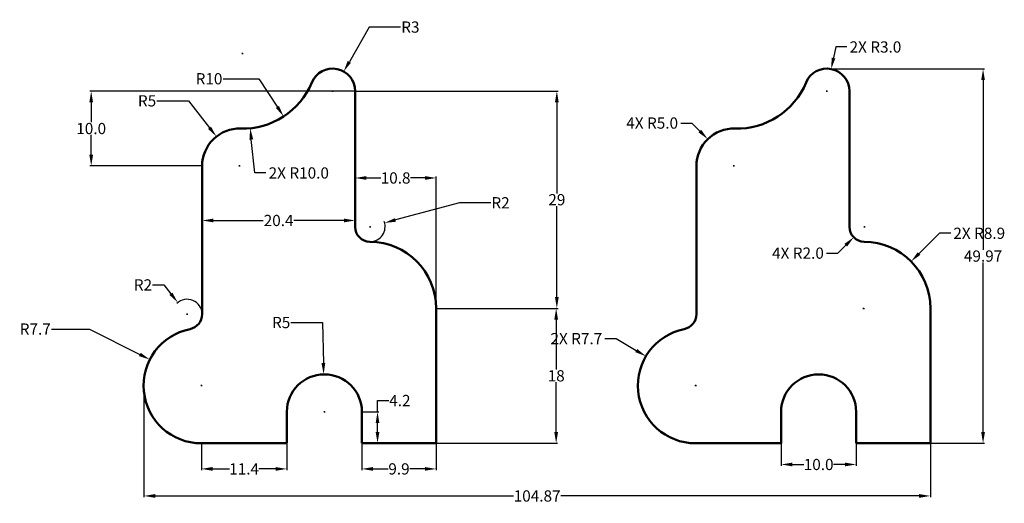
# Model space of a CAD drawing. Units: millimetres. Extents: x -11 to 121, y -3 to 61.
import ezdxf

# ---------------------------------------------------------------- set-up
doc = ezdxf.new("R2010")
doc.units = ezdxf.units.MM
doc.header["$MEASUREMENT"] = 0
doc.layers.add('M-DIMS', color=3, linetype='Continuous', lineweight=25)
doc.layers.add('M-OUTL', color=7, linetype='Continuous', lineweight=50)
doc.styles.get("Standard").update_dxf_attribs({"font": 'arial.ttf'})
doc.dimstyles.get("Standard").update_dxf_attribs({"dimtxt": 1.5, "dimasz": 1.5, "dimexe": 0.18, "dimexo": 0.0625, "dimgap": 0.09, "dimtad": 0, "dimtih": 1, "dimtoh": 1, "dimdec": 1, "dimdsep": 46, "dimtxsty": 'Standard', "dimcen": 0.09, "dimadec": 0, "dimazin": 0, "dimtfac": 1, "dimtdec": 1, "dimtofl": 0, "dimtmove": 0, "dimatfit": 3, "dimfxl": 1, "dimtolj": 1, "dimtzin": 0, "dimarcsym": 0})

# ---------------------------------------------------------------- blocks, each defined once
blk = doc.blocks.new('*D1')
at = {"layer": 'Defpoints', "color": 0, "transparency": 16777216}
for p in [(13.55, 4.95), (24.95, 4.95), (24.95, 1.53)]:
    blk.add_point(p, dxfattribs=at)
at = {"layer": 'M-DIMS', "color": 0, "lineweight": -2, "transparency": 16777216}
for p, q in [((13.55, 4.88), (13.55, 1.35)), ((24.95, 4.88), (24.95, 1.35)), ((15.05, 1.53), (17.29, 1.53)), ((23.45, 1.53), (21.22, 1.53))]:
    blk.add_line(p, q, dxfattribs=at)
at = {"layer": 'M-DIMS', "color": 0, "transparency": 16777216}
for points in [[(15.05, 1.78), (15.05, 1.28), (13.55, 1.53)], [(23.45, 1.78), (23.45, 1.28), (24.95, 1.53)]]:
    blk.add_solid(points, dxfattribs=at)
at = {"layer": 'M-DIMS', "color": 0, "transparency": 16777216, "insert": (19.25, 1.53), "char_height": 1.5, "attachment_point": 5}
blk.add_mtext('\\A1;11.4', dxfattribs=at)
blk = doc.blocks.new('*D2')
at = {"layer": 'Defpoints', "color": 0, "transparency": 16777216}
for p in [(34.95, 4.95), (44.85, 4.95), (44.85, 1.53)]:
    blk.add_point(p, dxfattribs=at)
at = {"layer": 'M-DIMS', "color": 0, "lineweight": -2, "transparency": 16777216}
for p, q in [((34.95, 4.88), (34.95, 1.35)), ((44.85, 4.88), (44.85, 1.35)), ((36.45, 1.53), (38.44, 1.53)), ((43.35, 1.53), (41.36, 1.53))]:
    blk.add_line(p, q, dxfattribs=at)
at = {"layer": 'M-DIMS', "color": 0, "transparency": 16777216}
for points in [[(36.45, 1.78), (36.45, 1.28), (34.95, 1.53)], [(43.35, 1.78), (43.35, 1.28), (44.85, 1.53)]]:
    blk.add_solid(points, dxfattribs=at)
at = {"layer": 'M-DIMS', "color": 0, "transparency": 16777216, "insert": (39.9, 1.53), "char_height": 1.5, "attachment_point": 5}
blk.add_mtext('\\A1;9.9', dxfattribs=at)
blk = doc.blocks.new('*D3')
at = {"layer": 'Defpoints', "color": 0, "transparency": 16777216}
for p in [(34.95, 9.15), (37.04, 9.15), (34.95, 4.95)]:
    blk.add_point(p, dxfattribs=at)
at = {"layer": 'M-DIMS', "color": 0, "lineweight": -2, "transparency": 16777216}
for p, q in [((37.04, 9.15), (37.04, 10.65)), ((37.04, 10.65), (38.54, 10.65)), ((35.01, 9.15), (37.22, 9.15)), ((37.04, 6.45), (37.04, 7.65)), ((35.01, 4.95), (37.22, 4.95))]:
    blk.add_line(p, q, dxfattribs=at)
at = {"layer": 'M-DIMS', "color": 0, "transparency": 16777216}
for points in [[(36.79, 7.65), (37.29, 7.65), (37.04, 9.15)], [(36.79, 6.45), (37.29, 6.45), (37.04, 4.95)]]:
    blk.add_solid(points, dxfattribs=at)
at = {"layer": 'M-DIMS', "color": 0, "transparency": 16777216, "insert": (40.02, 10.65), "char_height": 1.5, "attachment_point": 5}
blk.add_mtext('\\A1;4.2', dxfattribs=at)
blk = doc.blocks.new('*D4')
at = {"layer": 'Defpoints', "color": 0, "transparency": 16777216}
for p in [(29.85, 14.15), (29.95, 9.15)]:
    blk.add_point(p, dxfattribs=at)
at = {"layer": 'M-DIMS', "color": 0, "lineweight": -2, "transparency": 16777216}
for p, q in [((25.5, 21.06), (29.71, 21.06)), ((29.71, 21.06), (29.82, 15.64)), ((29.95, 9.06), (29.95, 9.24)), ((29.86, 9.15), (30.04, 9.15))]:
    blk.add_line(p, q, dxfattribs=at)
at = {"layer": 'M-DIMS', "color": 0, "transparency": 16777216}
blk.add_solid([(30.07, 15.65), (29.57, 15.64), (29.85, 14.15)], dxfattribs=at)
at = {"layer": 'M-DIMS', "color": 0, "transparency": 16777216, "insert": (24.19, 21.06), "char_height": 1.5, "attachment_point": 5}
blk.add_mtext('\\A1;R5', dxfattribs=at)
blk = doc.blocks.new('*D5')
at = {"layer": 'Defpoints', "color": 0, "transparency": 16777216}
for p in [(6.68, 16.12), (13.55, 12.65)]:
    blk.add_point(p, dxfattribs=at)
at = {"layer": 'M-DIMS', "color": 0, "lineweight": -2, "transparency": 16777216}
for p, q in [((-6.43, 20.19), (-1.35, 20.19)), ((-1.35, 20.19), (5.34, 16.8)), ((13.46, 12.65), (13.64, 12.65)), ((13.55, 12.56), (13.55, 12.74))]:
    blk.add_line(p, q, dxfattribs=at)
at = {"layer": 'M-DIMS', "color": 0, "transparency": 16777216}
blk.add_solid([(5.46, 17.02), (5.23, 16.58), (6.68, 16.12)], dxfattribs=at)
at = {"layer": 'M-DIMS', "color": 0, "transparency": 16777216, "insert": (-8.6, 20.19), "char_height": 1.5, "attachment_point": 5}
blk.add_mtext('\\A1;R7.7', dxfattribs=at)
blk = doc.blocks.new('*D6')
at = {"layer": 'Defpoints', "color": 0, "transparency": 16777216}
for p in [(44.85, 22.95), (60.86, 22.95), (44.85, 4.95)]:
    blk.add_point(p, dxfattribs=at)
at = {"layer": 'M-DIMS', "color": 0, "lineweight": -2, "transparency": 16777216}
for p, q in [((44.91, 22.95), (61.04, 22.95)), ((60.86, 21.45), (60.86, 14.8)), ((60.86, 6.45), (60.86, 13.09)), ((44.91, 4.95), (61.04, 4.95))]:
    blk.add_line(p, q, dxfattribs=at)
at = {"layer": 'M-DIMS', "color": 0, "transparency": 16777216}
for points in [[(60.61, 21.45), (61.11, 21.45), (60.86, 22.95)], [(60.61, 6.45), (61.11, 6.45), (60.86, 4.95)]]:
    blk.add_solid(points, dxfattribs=at)
at = {"layer": 'M-DIMS', "color": 0, "transparency": 16777216, "insert": (60.86, 13.95), "char_height": 1.5, "attachment_point": 5}
blk.add_mtext('\\A1;18', dxfattribs=at)
blk = doc.blocks.new('*D7')
at = {"layer": 'Defpoints', "color": 0, "transparency": 16777216}
for p in [(34.05, 51.95), (60.95, 51.95), (44.85, 22.95)]:
    blk.add_point(p, dxfattribs=at)
at = {"layer": 'M-DIMS', "color": 0, "lineweight": -2, "transparency": 16777216}
for p, q in [((34.11, 51.95), (61.13, 51.95)), ((60.95, 50.45), (60.95, 38.3)), ((60.95, 24.45), (60.95, 36.59)), ((44.91, 22.95), (61.13, 22.95))]:
    blk.add_line(p, q, dxfattribs=at)
at = {"layer": 'M-DIMS', "color": 0, "transparency": 16777216}
for points in [[(60.7, 50.45), (61.2, 50.45), (60.95, 51.95)], [(60.7, 24.45), (61.2, 24.45), (60.95, 22.95)]]:
    blk.add_solid(points, dxfattribs=at)
at = {"layer": 'M-DIMS', "color": 0, "transparency": 16777216, "insert": (60.95, 37.45), "char_height": 1.5, "attachment_point": 5}
blk.add_mtext('\\A1;29', dxfattribs=at)
blk = doc.blocks.new('*D8')
at = {"layer": 'Defpoints', "color": 0, "transparency": 16777216}
for p in [(34.05, 40.35), (34.05, 33.85), (44.85, 22.95)]:
    blk.add_point(p, dxfattribs=at)
at = {"layer": 'M-DIMS', "color": 0, "lineweight": -2, "transparency": 16777216}
for p, q in [((34.05, 33.91), (34.05, 40.53)), ((35.55, 40.35), (37.48, 40.35)), ((43.35, 40.35), (41.42, 40.35)), ((44.85, 23.01), (44.85, 40.53))]:
    blk.add_line(p, q, dxfattribs=at)
at = {"layer": 'M-DIMS', "color": 0, "transparency": 16777216}
for points in [[(35.55, 40.6), (35.55, 40.1), (34.05, 40.35)], [(43.35, 40.6), (43.35, 40.1), (44.85, 40.35)]]:
    blk.add_solid(points, dxfattribs=at)
at = {"layer": 'M-DIMS', "color": 0, "transparency": 16777216, "insert": (39.45, 40.35), "char_height": 1.5, "attachment_point": 5}
blk.add_mtext('\\A1;10.8', dxfattribs=at)
blk = doc.blocks.new('*D9')
at = {"layer": 'Defpoints', "color": 0, "transparency": 16777216}
for p in [(34.05, 42.9), (13.65, 41.95), (13.65, 34.68)]:
    blk.add_point(p, dxfattribs=at)
at = {"layer": 'M-DIMS', "color": 0, "lineweight": -2, "transparency": 16777216}
for p, q in [((34.05, 42.83), (34.05, 34.5)), ((13.65, 41.88), (13.65, 34.5)), ((15.15, 34.68), (21.8, 34.68)), ((32.55, 34.68), (25.9, 34.68))]:
    blk.add_line(p, q, dxfattribs=at)
at = {"layer": 'M-DIMS', "color": 0, "transparency": 16777216}
for points in [[(15.15, 34.93), (15.15, 34.43), (13.65, 34.68)], [(32.55, 34.93), (32.55, 34.43), (34.05, 34.68)]]:
    blk.add_solid(points, dxfattribs=at)
at = {"layer": 'M-DIMS', "color": 0, "transparency": 16777216, "insert": (23.85, 34.68), "char_height": 1.5, "attachment_point": 5}
blk.add_mtext('\\A1;20.4', dxfattribs=at)
blk = doc.blocks.new('*D10')
at = {"layer": 'Defpoints', "color": 0, "transparency": 16777216}
for p in [(10.41, 23.73), (11.65, 22.16)]:
    blk.add_point(p, dxfattribs=at)
at = {"layer": 'M-DIMS', "color": 0, "lineweight": -2, "transparency": 16777216}
for p, q in [((7.05, 26.08), (8.55, 26.08)), ((8.55, 26.08), (9.48, 24.91)), ((11.56, 22.16), (11.74, 22.16)), ((11.65, 22.07), (11.65, 22.25))]:
    blk.add_line(p, q, dxfattribs=at)
blk.add_arc((11.65, 22.16), 2, 1.7905, 133.4184, dxfattribs=at)
at = {"layer": 'M-DIMS', "color": 0, "transparency": 16777216}
blk.add_solid([(9.68, 25.06), (9.29, 24.75), (10.41, 23.73)], dxfattribs=at)
at = {"layer": 'M-DIMS', "color": 0, "transparency": 16777216, "insert": (5.76, 26.08), "char_height": 1.5, "attachment_point": 5}
blk.add_mtext('\\A1;R2', dxfattribs=at)
blk = doc.blocks.new('*D11')
at = {"layer": 'Defpoints', "color": 0, "transparency": 16777216}
for p in [(37.98, 34.36), (36.05, 33.85)]:
    blk.add_point(p, dxfattribs=at)
at = {"layer": 'M-DIMS', "color": 0, "lineweight": -2, "transparency": 16777216}
for p, q in [((47.95, 37.04), (39.43, 34.75)), ((52.15, 37.04), (47.95, 37.04)), ((35.96, 33.85), (36.14, 33.85)), ((36.05, 33.76), (36.05, 33.94))]:
    blk.add_line(p, q, dxfattribs=at)
blk.add_arc((36.05, 33.85), 2, 271.2648, 20.1728, dxfattribs=at)
at = {"layer": 'M-DIMS', "color": 0, "transparency": 16777216}
blk.add_solid([(39.37, 34.99), (39.5, 34.51), (37.98, 34.36)], dxfattribs=at)
at = {"layer": 'M-DIMS', "color": 0, "transparency": 16777216, "insert": (53.44, 37.04), "char_height": 1.5, "attachment_point": 5}
blk.add_mtext('\\A1;R2', dxfattribs=at)
blk = doc.blocks.new('*D12')
at = {"layer": 'Defpoints', "color": 0, "transparency": 16777216}
for p in [(15.56, 45.88), (18.65, 41.95)]:
    blk.add_point(p, dxfattribs=at)
at = {"layer": 'M-DIMS', "color": 0, "lineweight": -2, "transparency": 16777216}
for p, q in [((7.61, 50.64), (11.83, 50.64)), ((11.83, 50.64), (14.64, 47.06)), ((18.65, 41.86), (18.65, 42.04)), ((18.56, 41.95), (18.74, 41.95))]:
    blk.add_line(p, q, dxfattribs=at)
at = {"layer": 'M-DIMS', "color": 0, "transparency": 16777216}
blk.add_solid([(14.83, 47.21), (14.44, 46.9), (15.56, 45.88)], dxfattribs=at)
at = {"layer": 'M-DIMS', "color": 0, "transparency": 16777216, "insert": (6.31, 50.64), "char_height": 1.5, "attachment_point": 5}
blk.add_mtext('\\A1;R5', dxfattribs=at)
blk = doc.blocks.new('*D13')
at = {"layer": 'Defpoints', "color": 0, "transparency": 16777216}
for p in [(19.05, 56.94), (24.51, 48.57)]:
    blk.add_point(p, dxfattribs=at)
at = {"layer": 'M-DIMS', "color": 0, "lineweight": -2, "transparency": 16777216}
for p, q in [((16.45, 53.59), (21.23, 53.59)), ((21.23, 53.59), (23.69, 49.82))]:
    blk.add_line(p, q, dxfattribs=at)
at = {"layer": 'M-DIMS', "color": 0, "transparency": 16777216}
blk.add_solid([(23.9, 49.96), (23.49, 49.69), (24.51, 48.57)], dxfattribs=at)
at = {"layer": 'M-DIMS', "color": 0, "transparency": 16777216, "insert": (14.57, 53.59), "char_height": 1.5, "attachment_point": 5}
blk.add_mtext('\\A1;R10', dxfattribs=at)
blk = doc.blocks.new('*D14')
at = {"layer": 'Defpoints', "color": 0, "transparency": 16777216}
for p in [(32.53, 54.55), (31.05, 51.95)]:
    blk.add_point(p, dxfattribs=at)
at = {"layer": 'M-DIMS', "color": 0, "lineweight": -2, "transparency": 16777216}
for p, q in [((35.91, 60.49), (33.28, 55.86)), ((40.12, 60.49), (35.91, 60.49)), ((30.96, 51.95), (31.14, 51.95)), ((31.05, 51.86), (31.05, 52.04))]:
    blk.add_line(p, q, dxfattribs=at)
at = {"layer": 'M-DIMS', "color": 0, "transparency": 16777216}
blk.add_solid([(33.06, 55.98), (33.49, 55.73), (32.53, 54.55)], dxfattribs=at)
at = {"layer": 'M-DIMS', "color": 0, "transparency": 16777216, "insert": (41.42, 60.49), "char_height": 1.5, "attachment_point": 5}
blk.add_mtext('\\A1;R3', dxfattribs=at)
blk = doc.blocks.new('PLATE-CONTOURED')
for p, q in [((28.2, 28.9), (28.2, 47)), ((7.8, 17.21), (7.8, 37)), ((39, 0), (39, 18)), ((19.1, 0), (19.1, 4.2)), ((29.1, 4.2), (29.1, 0)), ((7.7, 0), (19.1, 0)), ((29.1, 0), (39, 0))]:
    blk.add_line(p, q)
for centre, radius, start, end in [((25.2, 47), 3, 0, 157.4053), ((13.2, 51.99), 10, 268.4803, 337.4053), ((12.8, 37), 5, 88.4803, 180), ((30.2, 28.9), 2, 180, 269.4743), ((30.1, 18), 8.9, 0, 89.4743), ((5.8, 17.21), 2, 281.2959, 0), ((7.7, 7.7), 7.7, 101.2959, 270), ((24.1, 4.2), 5, 0, 180)]:
    blk.add_arc(centre, radius, start, end)
blk = doc.blocks.new('*D16')
at = {"layer": 'Defpoints', "color": 0, "transparency": 16777216}
for p in [(5.89, 11.89), (110.76, 4.95), (110.76, -2.08)]:
    blk.add_point(p, dxfattribs=at)
at = {"layer": 'M-DIMS', "color": 0, "lineweight": -2, "transparency": 16777216}
for p, q in [((5.89, 11.83), (5.89, -2.26)), ((110.76, 4.88), (110.76, -2.26)), ((7.39, -2.08), (55.19, -2.08)), ((109.26, -2.08), (61.46, -2.08))]:
    blk.add_line(p, q, dxfattribs=at)
at = {"layer": 'M-DIMS', "color": 0, "transparency": 16777216}
for points in [[(7.39, -1.83), (7.39, -2.33), (5.89, -2.08)], [(109.26, -1.83), (109.26, -2.33), (110.76, -2.08)]]:
    blk.add_solid(points, dxfattribs=at)
at = {"layer": 'M-DIMS', "color": 0, "transparency": 16777216, "insert": (58.32, -2.08), "char_height": 1.5, "attachment_point": 5}
blk.add_mtext('\\A1;104.87', dxfattribs=at)
blk = doc.blocks.new('*D17')
at = {"layer": 'Defpoints', "color": 0, "transparency": 16777216}
for p in [(90.856424, 9.146014), (100.856424, 9.146014), (90.856424, 2.121014)]:
    blk.add_point(p, dxfattribs=at)
at = {"layer": 'M-DIMS', "color": 0, "lineweight": -2, "transparency": 16777216}
for p, q in [((90.856424, 9.083514), (90.856424, 1.941014)), ((100.856424, 9.083514), (100.856424, 1.941014)), ((92.356424, 2.121014), (93.891424, 2.121014)), ((99.356424, 2.121014), (97.821424, 2.121014))]:
    blk.add_line(p, q, dxfattribs=at)
at = {"layer": 'M-DIMS', "color": 0, "transparency": 16777216}
for points in [[(92.356424, 2.371014), (92.356424, 1.871014), (90.856424, 2.121014)], [(99.356424, 2.371014), (99.356424, 1.871014), (100.856424, 2.121014)]]:
    blk.add_solid(points, dxfattribs=at)
at = {"layer": 'M-DIMS', "color": 0, "transparency": 16777216, "insert": (95.856424, 2.121014), "char_height": 1.5, "attachment_point": 5}
blk.add_mtext('\\A1;10.0', dxfattribs=at)
blk = doc.blocks.new('*D18')
at = {"layer": 'Defpoints', "color": 0, "transparency": 16777216}
for p in [(-1.14, 51.95), (34.05, 51.95), (13.65, 41.95)]:
    blk.add_point(p, dxfattribs=at)
at = {"layer": 'M-DIMS', "color": 0, "lineweight": -2, "transparency": 16777216}
for p, q in [((33.99, 51.95), (-1.32, 51.95)), ((-1.14, 50.45), (-1.14, 47.8)), ((-1.14, 43.45), (-1.14, 46.09)), ((13.59, 41.95), (-1.32, 41.95))]:
    blk.add_line(p, q, dxfattribs=at)
at = {"layer": 'M-DIMS', "color": 0, "transparency": 16777216}
for points in [[(-1.39, 50.45), (-0.89, 50.45), (-1.14, 51.95)], [(-1.39, 43.45), (-0.89, 43.45), (-1.14, 41.95)]]:
    blk.add_solid(points, dxfattribs=at)
at = {"layer": 'M-DIMS', "color": 0, "transparency": 16777216, "insert": (-1.14, 46.95), "char_height": 1.5, "attachment_point": 5}
blk.add_mtext('\\A1;10.0', dxfattribs=at)
blk = doc.blocks.new('*D19')
at = {"layer": 'Defpoints', "color": 0, "transparency": 16777216}
for p in [(96.51, 54.91), (117.78, 54.91), (110.76, 4.95)]:
    blk.add_point(p, dxfattribs=at)
at = {"layer": 'M-DIMS', "color": 0, "lineweight": -2, "transparency": 16777216}
for p, q in [((96.57, 54.91), (117.96, 54.91)), ((117.78, 53.41), (117.78, 30.78)), ((117.78, 6.45), (117.78, 29.07)), ((110.82, 4.95), (117.96, 4.95))]:
    blk.add_line(p, q, dxfattribs=at)
at = {"layer": 'M-DIMS', "color": 0, "transparency": 16777216}
for points in [[(117.53, 53.41), (118.03, 53.41), (117.78, 54.91)], [(117.53, 6.45), (118.03, 6.45), (117.78, 4.95)]]:
    blk.add_solid(points, dxfattribs=at)
at = {"layer": 'M-DIMS', "color": 0, "transparency": 16777216, "insert": (117.78, 29.93), "char_height": 1.5, "attachment_point": 5}
blk.add_mtext('\\A1;49.97', dxfattribs=at)
blk = doc.blocks.new('*D20')
at = {"layer": 'Defpoints', "color": 0, "transparency": 16777216}
for p in [(108.18, 29.21), (101.86, 22.95)]:
    blk.add_point(p, dxfattribs=at)
at = {"layer": 'M-DIMS', "color": 0, "lineweight": -2, "transparency": 16777216}
for p, q in [((111.97, 32.97), (109.24, 30.27)), ((113.47, 32.97), (111.97, 32.97)), ((101.77, 22.95), (101.95, 22.95)), ((101.86, 22.86), (101.86, 23.04))]:
    blk.add_line(p, q, dxfattribs=at)
at = {"layer": 'M-DIMS', "color": 0, "transparency": 16777216}
blk.add_solid([(109.07, 30.44), (109.42, 30.09), (108.18, 29.21)], dxfattribs=at)
at = {"layer": 'M-DIMS', "color": 0, "transparency": 16777216, "insert": (117.27, 32.97), "char_height": 1.5, "attachment_point": 5}
blk.add_mtext('\\A1;2X R8.9', dxfattribs=at)
blk = doc.blocks.new('*D21')
at = {"layer": 'Defpoints', "color": 0, "transparency": 16777216}
for p in [(72.83, 16.56), (79.46, 12.65)]:
    blk.add_point(p, dxfattribs=at)
at = {"layer": 'M-DIMS', "color": 0, "lineweight": -2, "transparency": 16777216}
for p, q in [((67.35, 18.91), (68.85, 18.91)), ((68.85, 18.91), (71.54, 17.33)), ((79.37, 12.65), (79.55, 12.65)), ((79.46, 12.56), (79.46, 12.74))]:
    blk.add_line(p, q, dxfattribs=at)
at = {"layer": 'M-DIMS', "color": 0, "transparency": 16777216}
blk.add_solid([(71.66, 17.54), (71.41, 17.11), (72.83, 16.56)], dxfattribs=at)
at = {"layer": 'M-DIMS', "color": 0, "transparency": 16777216, "insert": (63.55, 18.91), "char_height": 1.5, "attachment_point": 5}
blk.add_mtext('\\A1;2X R7.7', dxfattribs=at)
blk = doc.blocks.new('*D22')
at = {"layer": 'Defpoints', "color": 0, "transparency": 16777216}
for p in [(81.07, 45.53), (84.56, 41.95)]:
    blk.add_point(p, dxfattribs=at)
at = {"layer": 'M-DIMS', "color": 0, "lineweight": -2, "transparency": 16777216}
for p, q in [((77.47, 47.68), (78.97, 47.68)), ((78.97, 47.68), (80.02, 46.6)), ((84.56, 41.86), (84.56, 42.04)), ((84.47, 41.95), (84.65, 41.95))]:
    blk.add_line(p, q, dxfattribs=at)
at = {"layer": 'M-DIMS', "color": 0, "transparency": 16777216}
blk.add_solid([(80.2, 46.78), (79.84, 46.43), (81.07, 45.53)], dxfattribs=at)
at = {"layer": 'M-DIMS', "color": 0, "transparency": 16777216, "insert": (73.66, 47.68), "char_height": 1.5, "attachment_point": 5}
blk.add_mtext('\\A1;4X R5.0', dxfattribs=at)
blk = doc.blocks.new('*D23')
at = {"layer": 'Defpoints', "color": 0, "transparency": 16777216}
for p in [(97.54, 54.89), (96.96, 51.95)]:
    blk.add_point(p, dxfattribs=at)
at = {"layer": 'M-DIMS', "color": 0, "lineweight": -2, "transparency": 16777216}
for p, q in [((98.13, 57.83), (97.84, 56.36)), ((99.63, 57.83), (98.13, 57.83)), ((96.87, 51.95), (97.05, 51.95)), ((96.96, 51.86), (96.96, 52.04))]:
    blk.add_line(p, q, dxfattribs=at)
at = {"layer": 'M-DIMS', "color": 0, "transparency": 16777216}
blk.add_solid([(97.59, 56.41), (98.08, 56.31), (97.54, 54.89)], dxfattribs=at)
at = {"layer": 'M-DIMS', "color": 0, "transparency": 16777216, "insert": (103.43, 57.83), "char_height": 1.5, "attachment_point": 5}
blk.add_mtext('\\A1;2X R3.0', dxfattribs=at)
blk = doc.blocks.new('*D24')
at = {"layer": 'Defpoints', "color": 0, "transparency": 16777216}
for p in [(101.96, 33.85), (100.54, 32.44)]:
    blk.add_point(p, dxfattribs=at)
at = {"layer": 'M-DIMS', "color": 0, "lineweight": -2, "transparency": 16777216}
for p, q in [((101.87, 33.85), (102.05, 33.85)), ((101.96, 33.76), (101.96, 33.94)), ((96.91, 30.32), (98.41, 30.32)), ((98.41, 30.32), (99.47, 31.38))]:
    blk.add_line(p, q, dxfattribs=at)
at = {"layer": 'M-DIMS', "color": 0, "transparency": 16777216}
blk.add_solid([(99.3, 31.56), (99.65, 31.2), (100.54, 32.44)], dxfattribs=at)
at = {"layer": 'M-DIMS', "color": 0, "transparency": 16777216, "insert": (93.1, 30.32), "char_height": 1.5, "attachment_point": 5}
blk.add_mtext('\\A1;4X R2.0', dxfattribs=at)
blk = doc.blocks.new('*D25')
at = {"layer": 'Defpoints', "color": 0, "transparency": 16777216}
for p in [(19.05, 56.94), (20.06, 46.99)]:
    blk.add_point(p, dxfattribs=at)
at = {"layer": 'M-DIMS', "color": 0, "lineweight": -2, "transparency": 16777216}
for p, q in [((18.96, 56.94), (19.14, 56.94)), ((19.05, 56.85), (19.05, 57.03)), ((20.66, 41.02), (20.21, 45.5)), ((22.16, 41.02), (20.66, 41.02))]:
    blk.add_line(p, q, dxfattribs=at)
at = {"layer": 'M-DIMS', "color": 0, "transparency": 16777216}
blk.add_solid([(20.46, 45.52), (19.96, 45.47), (20.06, 46.99)], dxfattribs=at)
at = {"layer": 'M-DIMS', "color": 0, "transparency": 16777216, "insert": (26.54, 41.02), "char_height": 1.5, "attachment_point": 5}
blk.add_mtext('\\A1;2X R10.0', dxfattribs=at)

msp = doc.modelspace()

# ---------------------------------------------------------------- block references
at = {"layer": 'M-OUTL'}
for p in [(5.851, 4.946), (71.756, 4.946)]:
    msp.add_blockref('PLATE-CONTOURED', p, dxfattribs=at)

# ---------------------------------------------------------------- dimensions: what is measured, and where the dimension line sits
at = {"layer": 'M-DIMS', "transparency": 33554610}
for center, mpoint, picture, middle in [((31.051, 51.946), (32.534, 54.554), '*D14', (41.418, 60.489)), ((19.049, 56.941), (24.514, 48.566), '*D13', (14.566, 53.591)), ((18.651, 41.946), (15.564, 45.879), '*D12', (6.308, 50.637)), ((36.051, 33.846), (37.983, 34.364), '*D11', (53.443, 37.037)), ((13.551, 12.646), (6.681, 16.124), '*D5', (-8.605, 20.189)), ((29.951, 9.146), (29.851, 14.145), '*D4', (24.193, 21.061))]:
    dim = msp.add_radius_dim(center=center, mpoint=mpoint, dimstyle='Standard', override={"dimclrd": 0, "dimclre": 0, "dimclrt": 0}, dxfattribs=at)
    dim.commit()
    dim.dimension.update_dxf_attribs({"geometry": picture, "text_midpoint": middle, "dimtype": 164})
at = {"layer": 'M-DIMS'}
for center, mpoint, text, picture, middle in [((96.956, 51.946), (97.544, 54.888), '2X <>', '*D23', (103.427, 57.83)), ((101.956, 33.846), (100.538, 32.436), '4X <>', '*D24', (93.097, 30.321))]:
    dim = msp.add_radius_dim(center=center, mpoint=mpoint, text=text, dimstyle='Standard', override={"dimdec": 1, "dimlfac": 1, "dimrnd": 0, "dimzin": 0, "dimdsep": 46, "dimlunit": 2}, dxfattribs=at)
    dim.commit()
    dim.dimension.update_dxf_attribs({"geometry": picture, "text_midpoint": middle})
for center, mpoint, text, picture, middle in [((19.049, 56.941), (20.056, 46.992), '2X <>', '*D25', (26.537, 41.022)), ((84.556, 41.946), (81.068, 45.528), '4X <>', '*D22', (73.663, 47.677)), ((101.856, 22.946), (108.178, 29.21), '2X <>', '*D20', (117.271, 32.969)), ((79.456, 12.646), (72.827, 16.563), '2X <>', '*D21', (63.552, 18.914))]:
    dim = msp.add_radius_dim(center=center, mpoint=mpoint, text=text, dimstyle='Standard', override={"dimdec": 1, "dimlfac": 1, "dimrnd": 0, "dimzin": 0, "dimdsep": 46, "dimlunit": 2}, dxfattribs=at)
    dim.commit()
    dim.dimension.update_dxf_attribs({"geometry": picture, "text_midpoint": middle, "dimtype": 164})
for base, p1, p2, angle, override, picture, middle in [((117.781, 54.912), (110.756, 4.946), (96.505, 54.912), 90, {"dimdec": 2, "dimlfac": 1, "dimrnd": 0, "dimzin": 0, "dimdsep": 46, "dimlunit": 2}, '*D19', (117.781, 29.929)), ((-1.137, 51.946), (13.651, 41.946), (34.051, 51.946), 90, {"dimdec": 1, "dimlfac": 1, "dimrnd": 0, "dimzin": 0, "dimdsep": 46, "dimlunit": 2}, '*D18', (-1.137, 46.946)), ((90.856, 2.121), (100.856, 9.146), (90.856, 9.146), 180, {"dimdec": 1, "dimlfac": 1, "dimrnd": 0, "dimzin": 0, "dimdsep": 46, "dimlunit": 2}, '*D17', (95.856, 2.121))]:
    dim = msp.add_linear_dim(base=base, p1=p1, p2=p2, angle=angle, dimstyle='Standard', override=override, dxfattribs=at)
    dim.commit()
    dim.dimension.update_dxf_attribs({"geometry": picture, "text_midpoint": middle})
at = {"layer": 'M-DIMS', "transparency": 33554610}
for base, p1, p2, picture, middle in [((60.945, 51.946), (44.851, 22.946), (34.051, 51.946), '*D7', (60.945, 37.446)), ((60.862, 22.946), (44.851, 4.946), (44.851, 22.946), '*D6', (60.862, 13.946)), ((37.042, 9.146), (34.951, 4.946), (34.951, 9.146), '*D3', (40.02, 10.646))]:
    dim = msp.add_linear_dim(base=base, p1=p1, p2=p2, angle=90, dimstyle='Standard', override={"dimclrd": 0, "dimclre": 0, "dimclrt": 0}, dxfattribs=at)
    dim.commit()
    dim.dimension.update_dxf_attribs({"geometry": picture, "text_midpoint": middle})
for base, p1, p2, picture, middle in [((13.651, 34.683), (34.051, 42.896), (13.651, 41.946), '*D9', (23.851, 34.683)), ((34.051, 40.35), (44.851, 22.946), (34.051, 33.846), '*D8', (39.451, 40.35)), ((24.951, 1.532), (13.551, 4.946), (24.951, 4.946), '*D1', (19.251, 1.532)), ((44.851, 1.532), (34.951, 4.946), (44.851, 4.946), '*D2', (39.901, 1.532))]:
    dim = msp.add_linear_dim(base=base, p1=p1, p2=p2, dimstyle='Standard', override={"dimclrd": 0, "dimclre": 0, "dimclrt": 0}, dxfattribs=at)
    dim.commit()
    dim.dimension.update_dxf_attribs({"geometry": picture, "text_midpoint": middle})
dim = msp.add_radius_dim(center=(11.651, 22.158), mpoint=(10.413, 23.728), dimstyle='Standard', override={"dimclrd": 0, "dimclre": 0, "dimclrt": 0}, dxfattribs=at)
dim.commit()
dim.dimension.update_dxf_attribs({"geometry": '*D10', "text_midpoint": (5.763, 26.084)})
at = {"layer": 'M-DIMS'}
dim = msp.add_linear_dim(base=(110.756, -2.079), p1=(5.888, 11.888), p2=(110.756, 4.946), dimstyle='Standard', override={"dimdec": 2, "dimlfac": 1, "dimrnd": 0, "dimzin": 0, "dimdsep": 46, "dimlunit": 2}, dxfattribs=at)
dim.commit()
dim.dimension.update_dxf_attribs({"geometry": '*D16', "text_midpoint": (58.322, -2.079)})

doc.saveas('drawing.dxf')
